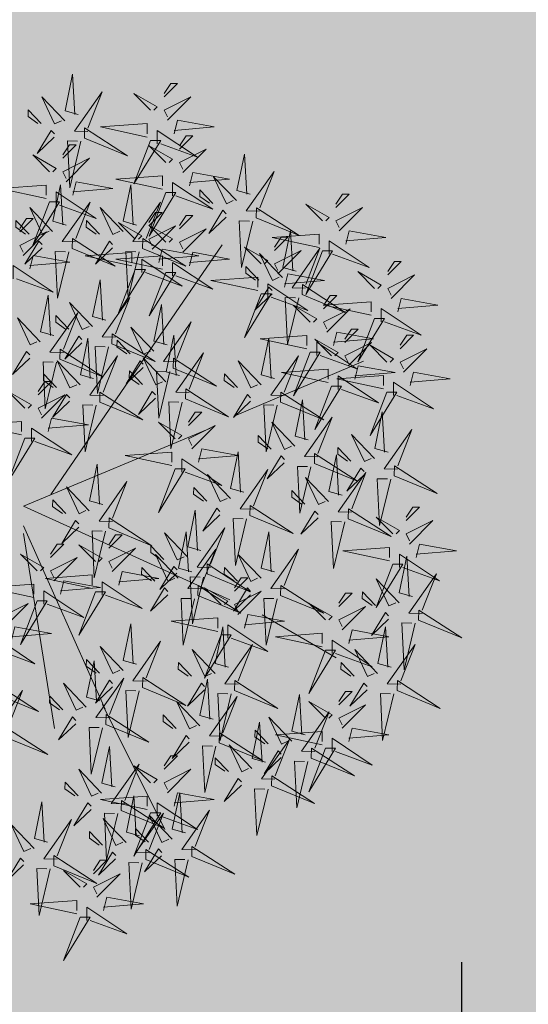
# Model space of a CAD drawing. Units: inches. Extents: x 1704 to 6393, y -157 to 1172.
# Tile 16 of 122: x 1912 to 1934, y 157 to 201. Entities that reach past the tile are written whole.
import ezdxf

# ---------------------------------------------------------------- set-up
doc = ezdxf.new("R2010")
doc.units = ezdxf.units.IN
doc.header["$MEASUREMENT"] = 0
doc.layers.add('A-ANNO-DIMS', color=7, linetype='Continuous', lineweight=13)
doc.layers.add('L-shrub', color=74, linetype='Continuous', lineweight=18)
doc.layers.add('L-PLNT-PATT', color=253, linetype='Continuous', lineweight=13, true_color=0x9abc8f)
doc.styles.get("Standard").update_dxf_attribs({"font": 'arial.ttf'})
doc.dimstyles.get("Standard").update_dxf_attribs({"dimtxt": 6, "dimasz": 2, "dimexe": 0.18, "dimexo": 0.0625, "dimgap": 0.09, "dimtad": 0, "dimtih": 1, "dimtoh": 1, "dimdec": 1, "dimzin": 0, "dimdsep": 46, "dimlunit": 3, "dimtxsty": 'Standard', "dimblk": 'ARCHTICK', "dimcen": 0.09, "dimadec": 0, "dimazin": 0, "dimtfac": 1, "dimtdec": 1, "dimtofl": 0, "dimtmove": 0, "dimatfit": 3, "dimfxl": 1, "dimtolj": 1, "dimtzin": 0, "dimarcsym": 0})

# ---------------------------------------------------------------- blocks, each defined once
blk = doc.blocks.new('shrub3')
for p, q in [((-68.47, 143.52), (-106.19, 232.32)), ((68.94, 162.35), (98.58, 213.48)), ((-5.99, -2.5), (58.67, 140.12)), ((-14.08, 16.34), (-186.51, 134.74)), ((-5.99, -2.5), (-59.88, 126.66)), ((130.91, 52.02), (217.13, 95.08)), ((7.48, -2.5), (134.11, 54.01)), ((12.87, -2.5), (147.58, 19.03))]:
    blk.add_line(p, q)
for points in [[(72.58, 270.39), (84.86, 300.11), (65.67, 270.57), (72.58, 270.39)], [(29.32, 268.76), (20.08, 271.07), (24.7, 296.43), (27.01, 268.76)], [(-89.4, 264.53), (-98.64, 266.83), (-94.02, 292.2), (-91.71, 264.53)], [(-140.28, 256.06), (-149.52, 258.36), (-144.9, 283.73), (-142.59, 256.06)], [(-82.48, 253), (-91.71, 253), (-73.24, 280.67), (-82.48, 255.31)], [(-27.06, 253.45), (-14.78, 283.17), (-33.97, 253.63), (-27.06, 253.45)], [(20.08, 264.15), (3.92, 280.29), (13.16, 261.85), (17.78, 264.15)], [(36.24, 257.23), (27.01, 257.23), (45.48, 284.9), (36.24, 259.54)], [(68.03, 272.82), (67.8, 263.59), (40.6, 282.74), (65.73, 272.87)], [(121.34, 255.57), (133.62, 285.29), (114.43, 255.75), (121.34, 255.57)], [(-133.36, 244.53), (-142.59, 244.53), (-124.12, 272.2), (-133.36, 246.84)], [(-98.64, 259.92), (-114.8, 276.06), (-105.56, 257.61), (-100.94, 259.92)], [(-149.52, 251.45), (-165.68, 267.59), (-156.44, 249.14), (-151.83, 251.45)], [(-114.8, 257.61), (-124.03, 266.83), (-124.03, 262.22), (-117.11, 257.61)], [(-31.61, 255.88), (-31.84, 246.65), (-59.04, 265.8), (-33.91, 255.94)], [(3.92, 261.85), (-5.31, 271.07), (-5.31, 266.46), (1.62, 261.85)], [(56.33, 266.18), (53.8, 257.01), (28.56, 262.26), (56.27, 263.87)], [(74.83, 268.03), (106.93, 260.3), (74.6, 258.8), (74.77, 265.72)], [(116.79, 258), (116.56, 248.76), (89.36, 267.92), (114.49, 258.05)], [(-165.68, 249.14), (-174.91, 258.36), (-174.91, 253.75), (-167.99, 249.14)], [(33.94, 252.62), (63.95, 241.09), (33.94, 259.54), (33.94, 252.62)], [(-105.56, 248.39), (-117.11, 236.86), (-107.87, 253), (-105.56, 250.69)], [(-93.64, 226.42), (-102.88, 228.72), (-98.26, 254.08), (-95.95, 226.42)], [(-84.78, 248.39), (-54.77, 236.86), (-84.78, 255.31), (-84.78, 248.39)], [(13.16, 252.62), (1.62, 241.09), (10.85, 257.23), (13.16, 254.93)], [(60.71, 256.84), (44.17, 241.08), (62.84, 249.85), (60.65, 254.53)], [(123.59, 253.21), (155.69, 245.48), (123.36, 243.97), (123.53, 250.9)], [(-186.92, 220.06), (-196.16, 222.37), (-191.54, 247.73), (-189.23, 220.06)], [(-135.66, 239.92), (-105.65, 228.39), (-135.66, 246.84), (-135.66, 239.92)], [(-87.09, 246.08), (-94.02, 213.8), (-96.33, 246.08), (-89.4, 246.08)], [(-43.31, 249.24), (-45.84, 240.07), (-71.08, 245.32), (-43.37, 246.93)], [(-24.81, 251.09), (7.29, 243.36), (-25.04, 241.86), (-24.87, 248.78)], [(2.62, 221.69), (14.9, 251.41), (-4.29, 221.87), (2.62, 221.69)], [(31.63, 250.32), (24.7, 218.04), (22.39, 250.32), (29.32, 250.32)], [(72.06, 249.62), (83.3, 237.79), (67.4, 247.43), (69.76, 249.68)], [(105.09, 251.36), (102.56, 242.19), (77.32, 247.44), (105.04, 249.05)], [(88.68, 222.18), (79.44, 224.49), (84.06, 249.85), (86.37, 222.18)], [(156.52, 222.18), (147.29, 224.49), (151.9, 249.85), (154.21, 222.18)], [(-156.44, 239.92), (-167.99, 228.39), (-158.75, 244.53), (-156.44, 242.22)], [(-116.96, 211.59), (-126.2, 213.9), (-121.58, 239.26), (-119.27, 211.59)], [(-86.72, 214.89), (-95.95, 214.89), (-77.48, 242.56), (-86.72, 217.19)], [(-38.93, 239.9), (-55.47, 224.14), (-36.8, 232.91), (-38.99, 237.59)], [(62.61, 240.62), (53.16, 231.62), (57.77, 231.51), (62.55, 238.31)], [(95.61, 210.65), (86.37, 210.65), (104.84, 238.32), (95.61, 212.96)], [(109.47, 242.01), (92.93, 226.26), (111.6, 235.03), (109.41, 239.71)], [(163.45, 210.65), (154.21, 210.65), (172.68, 238.32), (163.45, 212.96)], [(-196.16, 215.45), (-212.32, 231.59), (-203.08, 213.15), (-198.47, 215.45)], [(-180, 208.53), (-189.23, 208.53), (-170.76, 236.2), (-180, 210.84)], [(-137.97, 237.61), (-144.9, 205.33), (-147.21, 237.61), (-140.28, 237.61)], [(-102.88, 221.8), (-119.04, 237.94), (-109.8, 219.5), (-105.18, 221.8)], [(-27.58, 232.68), (-16.34, 220.86), (-32.24, 230.49), (-29.88, 232.74)], [(-1.93, 224.12), (-2.16, 214.89), (-29.36, 234.04), (-4.23, 224.17)], [(79.44, 217.57), (63.28, 233.71), (72.52, 215.26), (77.14, 217.57)], [(120.82, 234.8), (132.06, 222.97), (116.16, 232.61), (118.52, 234.86)], [(147.29, 217.57), (131.13, 233.71), (140.36, 215.26), (144.98, 217.57)], [(-119.04, 219.5), (-128.27, 228.72), (-128.27, 224.11), (-121.35, 219.5)], [(-110.04, 200.06), (-119.27, 200.06), (-100.8, 227.73), (-110.04, 202.37)], [(-35.54, 198.4), (-23.26, 228.12), (-42.45, 198.58), (-35.54, 198.4)], [(63.28, 215.26), (54.05, 224.49), (54.05, 219.87), (60.98, 215.26)], [(111.37, 225.8), (101.92, 216.8), (106.53, 216.68), (111.31, 223.49)], [(131.13, 215.26), (121.89, 224.49), (121.89, 219.87), (128.82, 215.26)], [(167.98, 196.29), (180.26, 226), (161.07, 196.46), (167.98, 196.29)], [(-212.32, 213.15), (-221.55, 222.37), (-221.55, 217.76), (-214.63, 213.15)], [(-152.14, 189.93), (-139.86, 219.65), (-159.05, 190.11), (-152.14, 189.93)], [(-126.2, 206.98), (-142.36, 223.12), (-133.12, 204.68), (-128.5, 206.98)], [(-37.03, 223.68), (-46.48, 214.68), (-41.87, 214.57), (-37.09, 221.37)], [(4.87, 219.33), (36.97, 211.6), (4.64, 210.1), (4.81, 217.02)], [(-182.31, 203.92), (-152.29, 192.39), (-182.31, 210.84), (-182.31, 203.92)], [(-142.36, 204.68), (-151.59, 213.9), (-151.59, 209.29), (-144.67, 204.68)], [(-109.8, 210.27), (-121.35, 198.75), (-112.11, 214.89), (-109.8, 212.58)], [(-89.02, 210.27), (-59.01, 198.75), (-89.02, 217.19), (-89.02, 210.27)], [(-13.63, 217.48), (-16.16, 208.31), (-41.4, 213.56), (-13.69, 215.17)], [(93.3, 206.04), (123.31, 194.51), (93.3, 212.96), (93.3, 206.04)], [(161.14, 206.04), (191.15, 194.51), (161.14, 212.96), (161.14, 206.04)], [(-203.08, 203.92), (-214.63, 192.39), (-205.39, 208.53), (-203.08, 206.23)], [(-157.24, 177.72), (-166.48, 180.02), (-161.86, 205.38), (-159.55, 177.72)], [(-91.33, 207.97), (-98.26, 175.69), (-100.57, 207.97), (-93.64, 207.97)], [(-77.94, 175.11), (-65.66, 204.83), (-84.85, 175.28), (-77.94, 175.11)], [(-40.09, 200.83), (-40.32, 191.59), (-67.52, 210.75), (-42.39, 200.88)], [(-9.25, 208.13), (-25.79, 192.38), (-7.12, 201.15), (-9.31, 205.83)], [(55.62, 175.11), (67.9, 204.83), (48.71, 175.28), (55.62, 175.11)], [(72.52, 206.04), (60.98, 194.51), (70.21, 210.65), (72.52, 208.35)], [(140.36, 206.04), (128.82, 194.51), (138.05, 210.65), (140.36, 208.35)], [(163.43, 198.71), (163.2, 189.48), (136, 208.63), (161.13, 198.77)], [(-184.61, 201.62), (-191.54, 169.34), (-193.85, 201.62), (-186.92, 201.62)], [(-156.69, 192.36), (-156.92, 183.12), (-184.12, 202.28), (-159, 192.41)], [(-133.12, 195.45), (-144.67, 183.92), (-135.43, 200.06), (-133.12, 197.76)], [(-112.34, 195.45), (-82.33, 183.92), (-112.34, 202.37), (-112.34, 195.45)], [(2.1, 200.92), (13.34, 189.09), (-2.56, 198.73), (-0.2, 200.98)], [(90.99, 203.73), (84.06, 171.45), (81.75, 203.73), (88.68, 203.73)], [(158.83, 203.73), (151.9, 171.45), (149.59, 203.73), (156.52, 203.73)], [(187.06, 168.76), (199.34, 198.47), (180.15, 168.93), (187.06, 168.76)], [(-150.32, 166.19), (-159.55, 166.19), (-141.08, 193.86), (-150.32, 168.49)], [(-114.65, 193.15), (-121.58, 160.87), (-123.89, 193.15), (-116.96, 193.15)], [(-51.79, 194.19), (-54.32, 185.02), (-79.56, 190.27), (-51.85, 191.88)], [(-33.29, 196.04), (-1.19, 188.31), (-33.52, 186.81), (-33.35, 193.73)], [(-7.35, 191.92), (-16.8, 182.92), (-12.19, 182.81), (-7.41, 189.61)], [(151.73, 192.07), (149.2, 182.9), (123.96, 188.15), (151.68, 189.77)], [(170.23, 193.92), (202.33, 186.19), (170, 184.69), (170.17, 191.61)], [(-205.14, 158.17), (-192.86, 187.89), (-212.05, 158.35), (-205.14, 158.17)], [(-168.39, 185.72), (-170.92, 176.55), (-196.16, 181.8), (-168.45, 183.41)], [(-166.48, 173.1), (-182.64, 189.24), (-173.4, 170.8), (-168.79, 173.1)], [(-149.89, 187.57), (-117.79, 179.84), (-150.12, 178.34), (-149.95, 185.26)], [(-82.49, 177.53), (-82.72, 168.3), (-109.92, 187.46), (-84.79, 177.59)], [(-47.41, 184.84), (-63.95, 169.09), (-45.28, 177.86), (-47.47, 182.54)], [(0.5, 153.94), (12.78, 183.65), (-6.41, 154.11), (0.5, 153.94)], [(51.07, 177.53), (50.84, 168.3), (23.64, 187.46), (48.77, 177.59)], [(-182.64, 170.8), (-191.87, 180.02), (-191.87, 175.41), (-184.95, 170.8)], [(-36.06, 177.63), (-24.82, 165.8), (-40.72, 175.44), (-38.36, 177.69)], [(78.08, 150.19), (68.84, 152.49), (73.46, 177.86), (75.77, 150.19)], [(156.11, 182.73), (139.57, 166.97), (158.24, 175.74), (156.05, 180.42)], [(182.51, 171.18), (182.28, 161.95), (155.08, 181.11), (180.21, 171.24)], [(-209.69, 160.6), (-209.92, 151.36), (-237.12, 170.52), (-212, 160.65)], [(-164.01, 176.37), (-180.55, 160.62), (-161.88, 169.39), (-164.07, 174.07)], [(-94.19, 170.9), (-96.72, 161.73), (-121.96, 166.98), (-94.25, 168.59)], [(-75.69, 172.75), (-43.59, 165.01), (-75.92, 163.51), (-75.75, 170.44)], [(39.37, 170.9), (36.84, 161.73), (11.6, 166.98), (39.31, 168.59)], [(57.87, 172.75), (89.97, 165.01), (57.64, 163.51), (57.81, 170.44)], [(121.34, 143.35), (133.62, 173.06), (114.43, 143.52), (121.34, 143.35)], [(167.46, 175.51), (178.7, 163.69), (162.8, 173.32), (165.16, 175.57)], [(-173.4, 161.57), (-184.95, 150.05), (-175.71, 166.19), (-173.4, 163.88)], [(-152.66, 169.16), (-141.42, 157.33), (-157.33, 166.97), (-154.96, 169.22)], [(-152.62, 161.57), (-122.61, 150.05), (-152.62, 168.49), (-152.62, 161.57)], [(-45.51, 168.63), (-54.96, 159.63), (-50.35, 159.51), (-45.57, 166.32)], [(-4.05, 156.36), (-4.28, 147.13), (-31.48, 166.28), (-6.35, 156.42)], [(85.01, 138.66), (75.77, 138.66), (94.24, 166.33), (85.01, 140.97)], [(170.81, 164.55), (168.28, 155.37), (143.04, 160.62), (170.76, 162.24)], [(158.01, 166.51), (148.56, 157.51), (153.17, 157.4), (157.96, 164.21)], [(189.31, 166.39), (221.41, 158.66), (189.08, 157.16), (189.25, 164.09)], [(-162.11, 160.16), (-171.56, 151.16), (-166.95, 151.04), (-162.17, 157.85)], [(-154.93, 159.27), (-161.86, 126.99), (-164.17, 159.27), (-157.24, 159.27)], [(-89.81, 161.55), (-106.35, 145.8), (-87.68, 154.57), (-89.87, 159.24)], [(43.75, 161.55), (27.21, 145.8), (45.88, 154.57), (43.69, 159.24)], [(68.84, 145.58), (52.68, 161.72), (61.92, 143.27), (66.54, 145.58)], [(157.38, 132.76), (169.66, 162.48), (150.47, 132.94), (157.38, 132.76)], [(-221.39, 153.96), (-223.93, 144.79), (-249.17, 150.04), (-221.45, 151.65)], [(-202.89, 155.81), (-170.79, 148.07), (-203.12, 146.57), (-202.95, 153.5)], [(-78.46, 154.34), (-67.22, 142.51), (-83.13, 152.15), (-80.76, 154.4)], [(-15.75, 149.73), (-18.28, 140.55), (-43.52, 145.8), (-15.81, 147.42)], [(2.75, 151.57), (34.85, 143.84), (2.52, 142.34), (2.69, 149.26)], [(40.78, 124.29), (53.06, 154.01), (33.87, 124.47), (40.78, 124.29)], [(52.68, 143.27), (43.45, 152.49), (43.45, 147.88), (50.38, 143.27)], [(55.1, 154.34), (66.34, 142.51), (50.44, 152.15), (52.8, 154.4)], [(116.79, 145.77), (116.56, 136.54), (89.36, 155.7), (114.49, 145.83)], [(175.19, 155.2), (158.65, 139.45), (177.32, 148.22), (175.13, 152.89)], [(-217.01, 144.61), (-233.55, 128.86), (-214.88, 137.63), (-217.07, 142.31)], [(-87.91, 145.34), (-97.36, 136.34), (-92.75, 136.22), (-87.97, 143.03)], [(-36.4, 118.43), (-45.64, 120.73), (-41.02, 146.1), (-38.71, 118.43)], [(45.65, 145.34), (36.2, 136.34), (40.81, 136.22), (45.59, 143.03)], [(55.62, 117.94), (67.9, 147.66), (48.71, 118.11), (55.62, 117.94)], [(152.83, 135.19), (152.6, 125.95), (125.4, 145.11), (150.53, 135.24)], [(186.54, 147.99), (197.78, 136.16), (181.88, 145.8), (184.24, 148.05)], [(235.82, 113.71), (248.1, 143.42), (228.91, 113.88), (235.82, 113.71)], [(-227.2, 112.08), (-236.44, 114.38), (-231.82, 139.75), (-229.51, 112.08)], [(-205.66, 137.4), (-194.42, 125.57), (-210.33, 135.21), (-207.96, 137.46)], [(-172.08, 112.08), (-181.32, 114.38), (-176.7, 139.75), (-174.39, 112.08)], [(-80.06, 109.47), (-67.78, 139.19), (-86.97, 109.65), (-80.06, 109.47)], [(-11.37, 140.38), (-27.91, 124.63), (-9.24, 133.4), (-11.43, 138.07)], [(36.23, 126.72), (36, 117.49), (8.8, 136.64), (33.93, 126.77)], [(61.92, 134.05), (50.38, 122.52), (59.61, 138.66), (61.92, 136.35)], [(105.09, 139.14), (102.56, 129.96), (77.32, 135.21), (105.04, 136.83)], [(82.7, 134.05), (112.71, 122.52), (82.7, 140.97), (82.7, 134.05)], [(123.59, 140.98), (155.69, 133.25), (123.36, 131.75), (123.53, 138.68)], [(177.09, 138.99), (167.64, 129.99), (172.25, 129.87), (177.04, 136.68)], [(-101.26, 101), (-88.98, 130.72), (-108.17, 101.18), (-101.26, 101)], [(-45.64, 113.82), (-61.8, 129.96), (-52.56, 111.51), (-47.94, 113.82)], [(-29.48, 106.9), (-38.71, 106.9), (-20.24, 134.57), (-29.48, 109.2)], [(-0.02, 133.17), (11.22, 121.34), (-4.68, 130.97), (-2.32, 133.22)], [(51.07, 120.36), (50.84, 111.13), (23.64, 130.29), (48.77, 120.42)], [(80.39, 131.74), (73.46, 99.46), (71.15, 131.74), (78.08, 131.74)], [(109.47, 129.79), (92.93, 114.04), (111.6, 122.81), (109.41, 127.48)], [(159.63, 130.4), (191.73, 122.67), (159.4, 121.17), (159.57, 128.09)], [(-263.24, 101.49), (-272.48, 103.79), (-267.86, 129.16), (-265.55, 101.49)], [(-236.44, 107.46), (-252.6, 123.6), (-243.36, 105.16), (-238.75, 107.46)], [(-220.28, 100.55), (-229.51, 100.55), (-211.04, 128.22), (-220.28, 102.85)], [(-215.11, 128.4), (-224.56, 119.4), (-219.95, 119.28), (-215.17, 126.09)], [(-181.32, 107.46), (-197.48, 123.6), (-188.24, 105.16), (-183.63, 107.46)], [(-165.16, 100.55), (-174.39, 100.55), (-155.92, 128.22), (-165.16, 102.85)], [(-9.47, 124.17), (-18.92, 115.16), (-14.31, 115.05), (-9.53, 121.86)], [(141.13, 128.55), (138.6, 119.38), (113.36, 124.63), (141.08, 126.24)], [(120.82, 122.58), (132.06, 110.75), (116.16, 120.39), (118.52, 122.64)], [(201.04, 101.49), (191.81, 103.79), (196.42, 129.16), (198.73, 101.49)], [(231.27, 116.13), (231.04, 106.9), (203.84, 126.05), (228.97, 116.19)], [(-256.32, 89.96), (-265.55, 89.96), (-247.08, 117.63), (-256.32, 92.27)], [(-174.2, 90.9), (-183.44, 93.21), (-178.82, 118.57), (-176.51, 90.9)], [(-84.61, 111.9), (-84.84, 102.66), (-112.04, 121.82), (-86.91, 111.95)], [(-61.8, 111.51), (-71.03, 120.73), (-71.03, 116.12), (-64.1, 111.51)], [(24.53, 120.08), (22, 110.91), (-3.24, 116.16), (24.47, 117.77)], [(43.03, 121.93), (75.13, 114.2), (42.8, 112.7), (42.97, 119.62)], [(145.51, 119.2), (128.97, 103.45), (147.64, 112.22), (145.45, 116.9)], [(207.97, 89.96), (198.73, 89.96), (217.2, 117.63), (207.97, 92.27)], [(-272.48, 96.88), (-288.64, 113.02), (-279.4, 94.57), (-274.79, 96.88)], [(-252.6, 105.16), (-261.83, 114.38), (-261.83, 109.77), (-254.91, 105.16)], [(-197.48, 105.16), (-206.71, 114.38), (-206.71, 109.77), (-199.79, 105.16)], [(-183.94, 79.83), (-171.66, 109.54), (-190.85, 80), (-183.94, 79.83)], [(-105.81, 103.43), (-106.04, 94.19), (-133.24, 113.35), (-108.11, 103.48)], [(-31.78, 102.29), (-1.77, 90.76), (-31.78, 109.2), (-31.78, 102.29)], [(39.37, 113.73), (36.84, 104.56), (11.6, 109.81), (39.31, 111.42)], [(28.91, 110.73), (12.37, 94.98), (31.04, 103.75), (28.85, 108.43)], [(57.87, 115.58), (89.97, 107.84), (57.64, 106.34), (57.81, 113.27)], [(111.37, 113.58), (101.92, 104.58), (106.53, 104.46), (111.31, 111.27)], [(119.22, 79.83), (131.5, 109.54), (112.31, 80), (119.22, 79.83)], [(156.86, 111.99), (168.1, 100.16), (152.2, 109.8), (154.56, 112.05)], [(191.81, 96.88), (175.65, 113.02), (184.88, 94.57), (189.5, 96.88)], [(219.57, 109.49), (217.04, 100.32), (191.8, 105.57), (219.52, 107.19)], [(237.94, 81.95), (250.22, 111.66), (231.03, 82.12), (237.94, 81.95)], [(238.07, 111.34), (270.17, 103.61), (237.84, 102.11), (238.01, 109.03)], [(-288.64, 94.57), (-297.87, 103.79), (-297.87, 99.18), (-290.95, 94.57)], [(-222.59, 95.94), (-192.57, 84.41), (-222.59, 102.85), (-222.59, 95.94)], [(-183.44, 86.29), (-199.6, 102.43), (-190.36, 83.98), (-185.75, 86.29)], [(-167.28, 79.37), (-176.51, 79.37), (-158.04, 107.04), (-167.28, 81.68)], [(-167.46, 95.94), (-137.45, 84.41), (-167.46, 102.85), (-167.46, 95.94)], [(-96.31, 105.26), (-98.84, 96.09), (-124.08, 101.34), (-96.37, 102.95)], [(-77.81, 107.11), (-45.71, 99.37), (-78.04, 97.87), (-77.87, 104.8)], [(-52.56, 102.29), (-64.1, 90.76), (-54.87, 106.9), (-52.56, 104.59)], [(43.75, 104.38), (27.21, 88.63), (45.88, 97.4), (43.69, 102.07)], [(40.26, 103.52), (51.5, 91.69), (35.6, 101.33), (37.96, 103.58)], [(147.41, 102.99), (137.96, 93.99), (142.57, 93.88), (147.36, 100.68)], [(175.65, 94.57), (166.41, 103.79), (166.41, 99.18), (173.34, 94.57)], [(-243.36, 95.94), (-254.91, 84.41), (-245.67, 100.55), (-243.36, 98.24)], [(-188.24, 95.94), (-199.79, 84.41), (-190.55, 100.55), (-188.24, 98.24)], [(-117.51, 96.79), (-120.04, 87.62), (-145.28, 92.87), (-117.57, 94.48)], [(-91.93, 95.91), (-108.47, 80.16), (-89.8, 88.93), (-91.99, 93.61)], [(-99.01, 98.64), (-66.91, 90.91), (-99.24, 89.41), (-99.07, 96.33)], [(-34.09, 99.98), (-41.02, 67.7), (-43.33, 99.98), (-36.4, 99.98)], [(55.1, 97.17), (66.34, 85.34), (50.44, 94.98), (52.8, 97.23)], [(223.95, 100.15), (207.41, 84.4), (226.08, 93.17), (223.89, 97.84)], [(-279.4, 85.35), (-290.95, 73.82), (-281.71, 89.96), (-279.4, 87.65)], [(-258.63, 85.35), (-228.61, 73.82), (-258.63, 92.27), (-258.63, 85.35)], [(-224.89, 93.63), (-231.82, 61.35), (-234.13, 93.63), (-227.2, 93.63)], [(-188.49, 82.25), (-188.72, 73.02), (-215.92, 92.18), (-190.8, 82.31)], [(-199.6, 83.98), (-208.83, 93.21), (-208.83, 88.6), (-201.91, 83.98)], [(-169.77, 93.63), (-176.7, 61.35), (-179.01, 93.63), (-172.08, 93.63)], [(-80.58, 88.7), (-69.34, 76.87), (-85.25, 86.51), (-82.88, 88.76)], [(30.81, 94.52), (21.36, 85.52), (25.97, 85.41), (30.75, 92.21)], [(48.4, 63.38), (39.16, 65.68), (43.78, 91.04), (46.09, 63.38)], [(114.67, 82.25), (114.44, 73.02), (87.24, 92.18), (112.37, 82.31)], [(184.88, 85.35), (173.34, 73.82), (182.57, 89.96), (184.88, 87.65)], [(204.02, 65.01), (216.3, 94.72), (197.11, 65.18), (204.02, 65.01)], [(205.66, 85.35), (235.67, 73.82), (205.66, 92.27), (205.66, 85.35)], [(233.39, 84.37), (233.16, 75.14), (205.96, 94.29), (231.09, 84.43)], [(235.3, 92.94), (246.54, 81.11), (230.64, 90.74), (233, 92.99)], [(-260.93, 83.04), (-267.86, 50.76), (-270.17, 83.04), (-263.24, 83.04)], [(-169.58, 74.76), (-139.57, 63.23), (-169.58, 81.68), (-169.58, 74.76)], [(-113.13, 87.44), (-129.67, 71.69), (-111, 80.46), (-113.19, 85.14)], [(-118.22, 58.65), (-105.94, 88.37), (-125.13, 58.83), (-118.22, 58.65)], [(8.98, 56.54), (21.26, 86.25), (2.07, 56.71), (8.98, 56.54)], [(45.65, 88.17), (36.2, 79.17), (40.81, 79.05), (45.59, 85.86)], [(144.66, 54.42), (156.94, 84.13), (137.75, 54.59), (144.66, 54.42)], [(203.35, 83.04), (196.42, 50.76), (194.11, 83.04), (201.04, 83.04)], [(225.85, 83.93), (216.4, 74.93), (221.01, 74.82), (225.8, 81.63)], [(-200.19, 75.62), (-202.73, 66.44), (-227.97, 71.69), (-200.25, 73.31)], [(-190.36, 74.76), (-201.91, 63.23), (-192.67, 79.37), (-190.36, 77.07)], [(-181.69, 77.46), (-149.59, 69.73), (-181.92, 68.23), (-181.75, 75.15)], [(-101.78, 80.23), (-90.54, 68.4), (-106.45, 78.04), (-104.08, 80.29)], [(-90.03, 79.7), (-99.48, 70.7), (-94.87, 70.58), (-90.09, 77.39)], [(-77.94, 50.18), (-65.66, 79.9), (-84.85, 50.36), (-77.94, 50.18)], [(39.16, 58.76), (23, 74.9), (32.24, 56.46), (36.86, 58.76)], [(55.33, 51.85), (46.09, 51.85), (64.56, 79.52), (55.33, 54.15)], [(102.97, 75.62), (100.44, 66.44), (75.2, 71.69), (102.92, 73.31)], [(121.47, 77.46), (153.57, 69.73), (121.24, 68.23), (121.41, 75.15)], [(199.47, 67.43), (199.24, 58.2), (172.04, 77.35), (197.17, 67.49)], [(221.69, 77.73), (219.16, 68.56), (193.92, 73.81), (221.64, 75.43)], [(240.19, 79.58), (272.29, 71.85), (239.96, 70.35), (240.13, 77.27)], [(273.12, 52.79), (263.89, 55.09), (268.5, 80.46), (270.81, 52.79)], [(-260.26, 39.6), (-247.98, 69.31), (-267.17, 39.77), (-260.26, 39.6)], [(-171.89, 72.46), (-178.82, 40.17), (-181.13, 72.46), (-174.2, 72.46)], [(-122.77, 61.08), (-123, 51.85), (-150.2, 71), (-125.08, 61.14)], [(-111.23, 71.23), (-120.68, 62.23), (-116.07, 62.11), (-111.29, 68.92)], [(4.43, 58.96), (4.2, 49.73), (-23, 68.88), (2.13, 59.02)], [(226.07, 68.39), (209.53, 52.64), (228.2, 61.41), (226.01, 66.08)], [(280.05, 41.26), (270.81, 41.26), (289.28, 68.93), (280.05, 43.57)], [(-195.81, 66.27), (-212.35, 50.52), (-193.68, 59.29), (-195.87, 63.96)], [(-82.49, 52.61), (-82.72, 43.38), (-109.92, 62.53), (-84.79, 52.67)], [(23, 56.46), (13.77, 65.68), (13.77, 61.07), (20.7, 56.46)], [(107.35, 66.27), (90.81, 50.52), (109.48, 59.29), (107.29, 63.96)], [(140.11, 56.84), (139.88, 47.61), (112.68, 66.77), (137.81, 56.9)], [(206.27, 62.64), (238.37, 54.91), (206.04, 53.41), (206.21, 60.33)], [(237.42, 61.17), (248.66, 49.35), (232.76, 58.98), (235.12, 61.23)], [(263.89, 48.18), (247.73, 64.32), (256.96, 45.87), (261.58, 48.18)], [(-220.84, 31.61), (-230.08, 33.92), (-225.46, 59.28), (-223.15, 31.61)], [(-183.94, 31.13), (-171.66, 60.84), (-190.85, 31.3), (-183.94, 31.13)], [(-184.46, 59.06), (-173.22, 47.23), (-189.13, 56.86), (-186.76, 59.12)], [(-134.47, 54.44), (-137, 45.27), (-162.24, 50.52), (-134.53, 52.13)], [(-115.97, 56.29), (-83.87, 48.56), (-116.2, 47.06), (-116.03, 53.98)], [(118.7, 59.06), (129.94, 47.23), (114.04, 56.86), (116.4, 59.12)], [(187.77, 60.79), (185.24, 51.62), (160, 56.87), (187.72, 58.49)], [(247.73, 45.87), (238.49, 55.09), (238.49, 50.48), (245.42, 45.87)], [(-264.81, 42.02), (-265.04, 32.79), (-292.24, 51.95), (-267.12, 42.08)], [(-213.92, 20.09), (-223.15, 20.09), (-204.68, 47.76), (-213.92, 22.39)], [(-193.91, 50.06), (-203.36, 41.06), (-198.75, 40.94), (-193.97, 47.75)], [(-107.62, 22.66), (-95.34, 52.37), (-114.53, 22.83), (-107.62, 22.66)], [(-75.69, 47.82), (-43.59, 40.09), (-75.92, 38.59), (-75.75, 45.51)], [(-7.27, 52.33), (-9.8, 43.15), (-35.04, 48.4), (-7.33, 50.02)], [(11.23, 54.17), (43.33, 46.44), (11, 44.94), (11.17, 51.86)], [(32.24, 47.24), (20.7, 35.71), (29.93, 51.85), (32.24, 49.54)], [(54.76, 23.15), (45.52, 25.45), (50.14, 50.81), (52.45, 23.15)], [(53.02, 47.24), (83.03, 35.71), (53.02, 54.15), (53.02, 47.24)], [(109.25, 50.06), (99.8, 41.06), (104.41, 40.94), (109.19, 47.75)], [(128.41, 50.21), (125.88, 41.03), (100.64, 46.28), (128.36, 47.9)], [(146.91, 52.05), (179.01, 44.32), (146.68, 42.82), (146.85, 49.75)], [(192.15, 51.45), (175.61, 35.7), (194.28, 44.47), (192.09, 49.14)], [(227.97, 52.17), (218.52, 43.17), (223.13, 43.06), (227.92, 49.87)], [(242.18, 18.42), (254.46, 48.14), (235.27, 18.6), (242.18, 18.42)], [(-230.08, 27), (-246.24, 43.14), (-237, 24.7), (-232.39, 27)], [(-188.49, 33.55), (-188.72, 24.32), (-215.92, 43.48), (-190.8, 33.61)], [(-130.09, 45.1), (-146.63, 29.34), (-127.96, 38.11), (-130.15, 42.79)], [(-94.19, 45.97), (-96.72, 36.8), (-121.96, 42.05), (-94.25, 43.67)], [(-57.6, 14.68), (-66.84, 16.98), (-62.22, 42.34), (-59.91, 14.68)], [(-2.89, 42.98), (-19.43, 27.23), (-0.76, 36), (-2.95, 40.67)], [(50.71, 44.93), (43.78, 12.65), (41.47, 44.93), (48.4, 44.93)], [(132.79, 40.86), (116.25, 25.11), (134.92, 33.88), (132.73, 38.55)], [(203.5, 44.24), (214.74, 32.41), (198.84, 42.04), (201.2, 44.29)], [(256.96, 36.65), (245.42, 25.12), (254.65, 41.26), (256.96, 38.95)], [(277.74, 36.65), (307.75, 25.12), (277.74, 43.57), (277.74, 36.65)], [(-276.51, 35.39), (-279.05, 26.21), (-304.29, 31.46), (-276.57, 33.08)], [(-258.01, 37.23), (-225.91, 29.5), (-258.24, 28), (-258.07, 34.92)], [(-112.17, 25.08), (-112.4, 15.85), (-139.6, 35.01), (-114.47, 25.14)], [(-118.74, 37.88), (-107.5, 26.06), (-123.41, 35.69), (-121.04, 37.94)], [(-89.81, 36.63), (-106.35, 20.87), (-87.68, 29.64), (-89.87, 34.32)], [(8.46, 35.77), (19.7, 23.94), (3.8, 33.57), (6.16, 35.82)], [(45.52, 18.53), (29.36, 34.67), (38.6, 16.23), (43.22, 18.53)], [(61.69, 11.62), (52.45, 11.62), (70.92, 39.29), (61.69, 13.92)], [(194.05, 35.23), (184.6, 26.23), (189.21, 26.12), (194, 32.93)], [(275.43, 34.34), (268.5, 2.06), (266.19, 34.34), (273.12, 34.34)], [(-246.24, 24.7), (-255.47, 33.92), (-255.47, 29.31), (-248.55, 24.7)], [(-181.69, 28.76), (-149.59, 21.03), (-181.92, 19.53), (-181.75, 26.45)], [(-169.96, 1.97), (-179.2, 4.28), (-174.58, 29.64), (-172.27, 1.97)], [(-128.19, 28.88), (-137.64, 19.88), (-133.03, 19.77), (-128.25, 26.57)], [(-78.46, 29.41), (-67.22, 17.59), (-83.13, 27.22), (-80.76, 29.47)], [(-50.68, 3.15), (-59.91, 3.15), (-41.44, 30.82), (-50.68, 5.45)], [(144.14, 33.65), (155.38, 21.82), (139.48, 31.46), (141.84, 33.71)], [(237.63, 20.85), (237.4, 11.62), (210.2, 30.77), (235.33, 20.91)], [(-272.13, 26.04), (-288.67, 10.29), (-270, 19.06), (-272.19, 23.73)], [(-200.19, 26.92), (-202.73, 17.74), (-227.97, 22.99), (-200.25, 24.61)], [(-216.23, 15.47), (-186.21, 3.95), (-216.23, 22.39), (-216.23, 15.47)], [(-87.91, 20.41), (-97.36, 11.41), (-92.75, 11.3), (-87.97, 18.11)], [(-66.84, 10.06), (-83, 26.2), (-73.76, 7.76), (-69.14, 10.06)], [(-0.99, 26.77), (-10.44, 17.76), (-5.83, 17.65), (-1.05, 24.46)], [(29.36, 16.23), (20.13, 25.45), (20.13, 20.84), (27.06, 16.23)], [(134.69, 24.65), (125.24, 15.65), (129.85, 15.53), (134.63, 22.34)], [(-260.78, 18.83), (-249.54, 7), (-265.45, 16.63), (-263.08, 18.88)], [(-237, 15.47), (-248.55, 3.95), (-239.31, 20.09), (-237, 17.78)], [(-195.81, 17.57), (-212.35, 1.82), (-193.68, 10.59), (-195.87, 15.26)], [(-163.04, -9.56), (-172.27, -9.56), (-153.8, 18.11), (-163.04, -7.25)], [(-123.87, 18.45), (-126.4, 9.27), (-151.64, 14.52), (-123.93, 16.14)], [(-105.37, 20.29), (-73.27, 12.56), (-105.6, 11.06), (-105.43, 17.99)], [(-83, 7.76), (-92.23, 16.98), (-92.23, 12.37), (-85.3, 7.76)], [(59.38, 7), (89.39, -4.52), (59.38, 13.92), (59.38, 7)], [(86.56, -10.73), (77.32, -8.43), (81.94, 16.94), (84.25, -10.73)], [(153.14, -15.45), (165.42, 14.26), (146.23, -15.28), (153.14, -15.45)], [(225.93, 14.21), (223.4, 5.04), (198.16, 10.29), (225.88, 11.9)], [(244.43, 16.06), (276.53, 8.33), (244.2, 6.83), (244.37, 13.75)], [(-270.23, 9.83), (-279.68, 0.83), (-275.07, 0.71), (-270.29, 7.52)], [(-218.53, 13.17), (-225.46, -19.11), (-227.77, 13.17), (-220.84, 13.17)], [(-179.2, -2.64), (-195.36, 13.5), (-186.12, -4.95), (-181.51, -2.64)], [(-184.46, 10.36), (-173.22, -1.47), (-189.13, 8.16), (-186.76, 10.41)], [(-119.49, 9.1), (-136.03, -6.65), (-117.36, 2.12), (-119.55, 6.79)], [(38.6, 7), (27.06, -4.52), (36.29, 11.62), (38.6, 9.31)], [(123.46, -21.81), (135.74, 7.91), (116.55, -21.63), (123.46, -21.81)], [(-195.36, -4.95), (-204.59, 4.28), (-204.59, -0.33), (-197.67, -4.95)], [(-193.91, 1.36), (-203.36, -7.64), (-198.75, -7.76), (-193.97, -0.95)], [(-108.14, 1.89), (-96.9, -9.94), (-112.81, -0.3), (-110.44, 1.95)], [(-73.76, -1.46), (-85.3, -12.99), (-76.07, 3.15), (-73.76, 0.84)], [(-52.98, -1.46), (-22.97, -12.99), (-52.98, 5.45), (-52.98, -1.46)], [(57.07, 4.7), (50.14, -27.58), (47.83, 4.7), (54.76, 4.7)], [(77.32, -15.34), (61.16, 0.8), (70.4, -17.65), (75.02, -15.34)], [(93.49, -22.26), (84.25, -22.26), (102.72, 5.41), (93.49, -19.96)], [(230.31, 4.87), (213.77, -10.89), (232.44, -2.12), (230.25, 2.56)], [(-55.29, -3.77), (-62.22, -36.05), (-64.53, -3.77), (-57.6, -3.77)], [(148.59, -13.03), (148.36, -22.26), (121.16, -3.11), (146.29, -12.97)], [(241.66, -2.35), (252.9, -14.18), (237, -4.54), (239.36, -2.29)]]:
    blk.add_lwpolyline(points)
blk = doc.blocks.new('_ArchTick')
at = {"color": 0, "linetype": 'ByBlock', "const_width": 0.15}
blk.add_lwpolyline([(-0.5, -0.5), (0.5, 0.5)], dxfattribs=at)
blk = doc.blocks.new('*D74')
at = {"layer": 'A-ANNO-DIMS', "color": 0, "lineweight": -2, "transparency": 16777216}
for p, q in [((1890.878, 159.062), (1890.878, 152.884)), ((1931.278, 159.062), (1931.278, 152.884)), ((1890.878, 153.064), (1888.878, 153.064)), ((1931.278, 153.064), (1933.278, 153.064))]:
    blk.add_line(p, q, dxfattribs=at)
at = {"layer": 'Defpoints', "color": 0, "lineweight": -3, "transparency": 16777216}
for p in [(1890.878, 159.124), (1931.278, 159.124), (1931.278, 153.064)]:
    blk.add_point(p, dxfattribs=at)
at = {"layer": 'A-ANNO-DIMS', "color": 0, "lineweight": -2, "transparency": 16777216, "xscale": 2, "yscale": 2, "zscale": 2}
blk.add_blockref('_ArchTick', (1890.878, 153.064), dxfattribs=at)
at = {"layer": 'A-ANNO-DIMS', "color": 0, "lineweight": -2, "transparency": 16777216, "xscale": 2, "yscale": 2, "zscale": 2, "rotation": 180}
blk.add_blockref('_ArchTick', (1931.278, 153.064), dxfattribs=at)
at = {"layer": 'A-ANNO-DIMS', "color": 0, "transparency": 16777216, "insert": (1911.078, 153.064), "char_height": 6, "attachment_point": 5}
blk.add_mtext('\\A1;SHRUB 40', dxfattribs=at)
blk = doc.blocks.new('*D93')
at = {"layer": 'A-ANNO-DIMS', "color": 0, "lineweight": -2, "transparency": 16777216}
for p, q in [((2605.286, 895.213), (1829.698, 895.213)), ((1829.878, 895.213), (1829.878, 495.866)), ((1829.878, 90.213), (1829.878, 489.56)), ((2605.286, 90.213), (1829.698, 90.213))]:
    blk.add_line(p, q, dxfattribs=at)
at = {"layer": 'Defpoints', "color": 0, "lineweight": -3, "transparency": 16777216}
for p in [(2605.349, 895.213), (1829.878, 90.213), (2605.349, 90.213)]:
    blk.add_point(p, dxfattribs=at)
at = {"layer": 'A-ANNO-DIMS', "color": 0, "lineweight": -2, "transparency": 16777216, "xscale": 2, "yscale": 2, "zscale": 2}
for p, rotation in [((1829.878, 895.213), 90), ((1829.878, 90.213), 270)]:
    blk.add_blockref('_ArchTick', p, dxfattribs=dict(at, rotation=rotation))
at = {"layer": 'A-ANNO-DIMS', "color": 0, "transparency": 16777216, "insert": (1829.878, 492.713), "char_height": 6, "attachment_point": 5}
blk.add_mtext('\\A1;805', dxfattribs=at)

msp = doc.modelspace()

# ---------------------------------------------------------------- hatches: boundary and pattern name
at = {"layer": 'L-PLNT-PATT', "transparency": 33554643}
h = msp.add_hatch(color=256, dxfattribs=at)
h.dxf.hatch_style = 1
h.paths.add_polyline_path([(1975.349, 202.213), (1898.349, 202.213), (1898.349, -3.787), (1975.349, -3.787)])

# ---------------------------------------------------------------- block references
at = {"layer": 'L-shrub', "xscale": 0.0642956299502212, "yscale": 0.0642956299502212, "zscale": 0.0642956299502212, "rotation": 270}
msp.add_blockref('shrub3', (1911.983, 178.911), dxfattribs=at)

# ---------------------------------------------------------------- dimensions: what is measured, and where the dimension line sits
at = {"layer": 'A-ANNO-DIMS'}
dim = msp.add_linear_dim(base=(1829.878, 90.213), p1=(2605.349, 895.213), p2=(2605.349, 90.213), angle=90, dimstyle='Standard', override={"dimdec": 0, "dimlfac": 1, "dimrnd": 0, "dimzin": 0, "dimdsep": 46, "dimlunit": 2}, dxfattribs=at)
dim.commit()
dim.dimension.update_dxf_attribs({"geometry": '*D93', "text_midpoint": (1829.878, 492.713)})
dim = msp.add_linear_dim(base=(1931.278, 153.064), p1=(1890.878, 159.124), p2=(1931.278, 159.124), text='SHRUB <>', dimstyle='Standard', override={"dimdec": 0, "dimlfac": 1, "dimrnd": 0, "dimzin": 0, "dimdsep": 46, "dimlunit": 2}, dxfattribs=at)
dim.commit()
dim.dimension.update_dxf_attribs({"geometry": '*D74', "text_midpoint": (1911.078, 153.064)})

doc.saveas('drawing.dxf')
